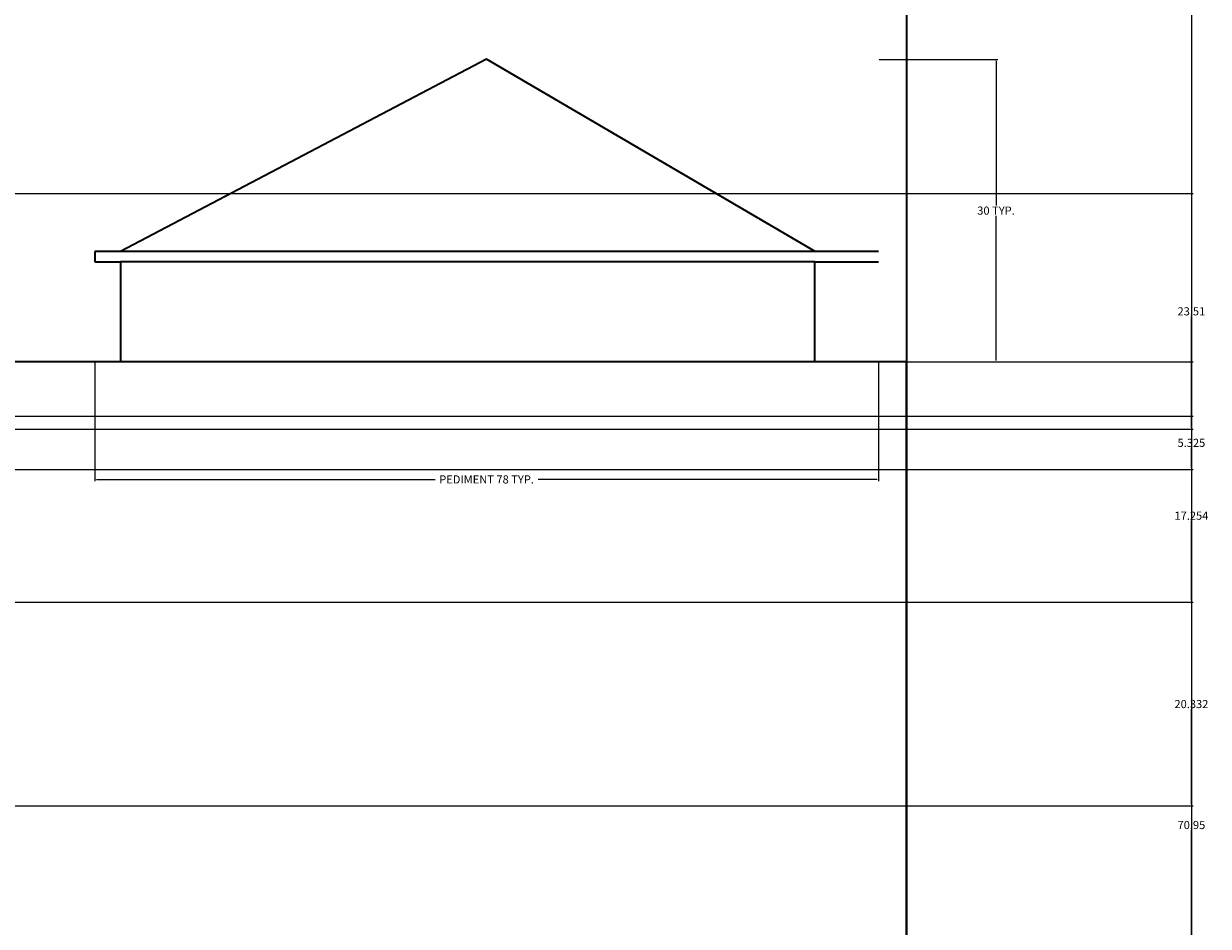
# Model space of a CAD drawing. Units: inches. Extents: x 69 to 650, y -16 to 573.
# Tile 22 of 26: x 531 to 650, y 308 to 398. Entities that reach past the tile are written whole.
import ezdxf

# ---------------------------------------------------------------- set-up
doc = ezdxf.new("R2010")
doc.units = ezdxf.units.IN
doc.header["$MEASUREMENT"] = 0
for name, color, linetype, lineweight in [('A-ANNO-DIMS', 2, 'Continuous', 18), ('A-ROOF', 7, 'Continuous', 35), ('A-WALL', 7, 'Continuous', 35)]:
    doc.layers.add(name, color=color, linetype=linetype, lineweight=lineweight)
doc.styles.get("Standard").update_dxf_attribs({"font": 'arial.ttf'})
doc.dimstyles.get("Standard").update_dxf_attribs({"dimtxt": 0.8125, "dimasz": 0.18, "dimexe": 0.18, "dimexo": 0.0625, "dimgap": 0.09, "dimtad": 0, "dimtih": 1, "dimtoh": 1, "dimdec": 4, "dimzin": 0, "dimdsep": 46, "dimlunit": 4, "dimtxsty": 'Standard', "dimcen": 0.09, "dimadec": 0, "dimazin": 0, "dimtfac": 1, "dimtdec": 4, "dimtofl": 0, "dimtmove": 0, "dimatfit": 3, "dimfxl": 1, "dimtolj": 1, "dimtzin": 0, "dimarcsym": 0})

# ---------------------------------------------------------------- blocks, each defined once
blk = doc.blocks.new('CAP-SIDE-PEDIMENT')
for p, q in [((39.09, 30.19), (2.58, 11)), ((71.85, 11), (39.09, 30.19)), ((78.18, 11), (0, 11)), ((0, 11), (0, 9.99)), ((0, 9.99), (2.58, 9.99)), ((71.82, 9.99), (2.58, 9.99)), ((2.58, 9.99), (2.58, 0)), ((71.82, 0), (71.82, 9.99)), ((71.82, 9.99), (78.18, 9.99))]:
    blk.add_line(p, q)
blk = doc.blocks.new('*D17')
at = {"layer": 'A-ANNO-DIMS', "color": 0, "lineweight": -2, "transparency": 16777216}
for p, q in [((538.56, 363.81), (538.56, 351.97)), ((616.75, 363.81), (616.75, 351.97)), ((538.74, 352.15), (572.52, 352.15)), ((616.57, 352.15), (582.79, 352.15))]:
    blk.add_line(p, q, dxfattribs=at)
at = {"layer": 'A-ANNO-DIMS', "color": 0, "transparency": 16777216}
for points in [[(538.74, 352.18), (538.74, 352.12), (538.56, 352.15)], [(616.57, 352.18), (616.57, 352.12), (616.75, 352.15)]]:
    blk.add_solid(points, dxfattribs=at)
at = {"layer": 'Defpoints', "color": 0, "transparency": 16777216}
for p in [(538.56, 363.87), (616.75, 363.87), (616.75, 352.15)]:
    blk.add_point(p, dxfattribs=at)
at = {"layer": 'A-ANNO-DIMS', "color": 0, "transparency": 16777216, "insert": (577.65, 352.15), "char_height": 0.8125, "attachment_point": 5}
blk.add_mtext('\\A1;PEDIMENT 78 TYP.', dxfattribs=at)
blk = doc.blocks.new('*D18')
at = {"layer": 'A-ANNO-DIMS', "color": 0, "lineweight": -2, "transparency": 16777216}
for p, q in [((616.81, 394.06), (628.65, 394.06)), ((628.47, 393.88), (628.47, 379.47)), ((628.47, 364.05), (628.47, 378.46)), ((616.81, 363.87), (628.65, 363.87))]:
    blk.add_line(p, q, dxfattribs=at)
at = {"layer": 'A-ANNO-DIMS', "color": 0, "transparency": 16777216}
for points in [[(628.44, 393.88), (628.5, 393.88), (628.47, 394.06)], [(628.44, 364.05), (628.5, 364.05), (628.47, 363.87)]]:
    blk.add_solid(points, dxfattribs=at)
at = {"layer": 'Defpoints', "color": 0, "transparency": 16777216}
for p in [(616.75, 394.06), (628.47, 394.06), (616.75, 363.87)]:
    blk.add_point(p, dxfattribs=at)
at = {"layer": 'A-ANNO-DIMS', "color": 0, "transparency": 16777216, "insert": (628.47, 378.97), "char_height": 0.8125, "attachment_point": 5}
blk.add_mtext('\\A1;30 TYP.', dxfattribs=at)
blk = doc.blocks.new('*D19')
at = {"layer": 'A-ANNO-DIMS', "color": 0, "lineweight": -2, "transparency": 16777216}
for p, q in [((99.56, 471.72), (99.56, 572.74)), ((99.74, 572.56), (358.57, 572.56)), ((619.38, 572.56), (360.54, 572.56)), ((619.56, 87.99), (619.56, 572.74))]:
    blk.add_line(p, q, dxfattribs=at)
at = {"layer": 'A-ANNO-DIMS', "color": 0, "transparency": 16777216}
for points in [[(99.74, 572.59), (99.74, 572.53), (99.56, 572.56)], [(619.38, 572.59), (619.38, 572.53), (619.56, 572.56)]]:
    blk.add_solid(points, dxfattribs=at)
at = {"layer": 'Defpoints', "color": 0, "transparency": 16777216}
for p in [(619.56, 572.56), (99.56, 471.66), (619.56, 87.93)]:
    blk.add_point(p, dxfattribs=at)
at = {"layer": 'A-ANNO-DIMS', "color": 0, "transparency": 16777216, "insert": (359.56, 572.56), "char_height": 0.812, "attachment_point": 5}
blk.add_mtext('\\A1;520', dxfattribs=at)
blk = doc.blocks.new('*D20')
at = {"layer": 'A-ANNO-DIMS', "color": 0, "lineweight": -2, "transparency": 16777216}
for p, q in [((504.24, 544.16), (648.14, 544.16)), ((647.96, 543.98), (647.96, 304.55)), ((647.96, 64.11), (647.96, 303.54)), ((619.62, 63.93), (648.14, 63.93))]:
    blk.add_line(p, q, dxfattribs=at)
at = {"layer": 'A-ANNO-DIMS', "color": 0, "transparency": 16777216}
for points in [[(647.93, 543.98), (647.99, 543.98), (647.96, 544.16)], [(647.93, 64.11), (647.99, 64.11), (647.96, 63.93)]]:
    blk.add_solid(points, dxfattribs=at)
at = {"layer": 'Defpoints', "color": 0, "transparency": 16777216}
for p in [(504.18, 544.16), (647.96, 544.16), (619.56, 63.93)]:
    blk.add_point(p, dxfattribs=at)
at = {"layer": 'A-ANNO-DIMS', "color": 0, "transparency": 16777216, "insert": (647.96, 304.04), "char_height": 0.812, "attachment_point": 5}
blk.add_mtext('\\A1;480.2', dxfattribs=at)
blk = doc.blocks.new('*D43')
at = {"layer": 'A-ANNO-DIMS', "color": 0, "lineweight": -2, "transparency": 16777216}
for p, q in [((502.63, 353.14), (648.14, 353.14)), ((647.96, 352.96), (647.96, 318.17)), ((647.96, 282.37), (647.96, 317.16)), ((502.63, 282.19), (648.14, 282.19))]:
    blk.add_line(p, q, dxfattribs=at)
at = {"layer": 'A-ANNO-DIMS', "color": 0, "transparency": 16777216}
for points in [[(647.93, 352.96), (647.99, 352.96), (647.96, 353.14)], [(647.93, 282.37), (647.99, 282.37), (647.96, 282.19)]]:
    blk.add_solid(points, dxfattribs=at)
at = {"layer": 'Defpoints', "color": 0, "transparency": 16777216}
for p in [(502.56, 353.14), (647.96, 353.14), (502.56, 282.19)]:
    blk.add_point(p, dxfattribs=at)
at = {"layer": 'A-ANNO-DIMS', "color": 0, "transparency": 16777216, "insert": (647.96, 317.67), "char_height": 0.812, "attachment_point": 5}
blk.add_mtext('\\A1;70.95', dxfattribs=at)
blk = doc.blocks.new('*D44')
at = {"layer": 'A-ANNO-DIMS', "color": 0, "lineweight": -2, "transparency": 16777216}
for p, q in [((470.47, 358.46), (648.14, 358.46)), ((647.96, 358.28), (647.96, 356.31)), ((647.96, 353.32), (647.96, 355.3)), ((502.63, 353.14), (648.14, 353.14))]:
    blk.add_line(p, q, dxfattribs=at)
at = {"layer": 'A-ANNO-DIMS', "color": 0, "transparency": 16777216}
for points in [[(647.93, 358.28), (647.99, 358.28), (647.96, 358.46)], [(647.93, 353.32), (647.99, 353.32), (647.96, 353.14)]]:
    blk.add_solid(points, dxfattribs=at)
at = {"layer": 'Defpoints', "color": 0, "transparency": 16777216}
for p in [(470.41, 358.46), (647.96, 358.46), (502.56, 353.14)]:
    blk.add_point(p, dxfattribs=at)
at = {"layer": 'A-ANNO-DIMS', "color": 0, "transparency": 16777216, "insert": (647.96, 355.8), "char_height": 0.812, "attachment_point": 5}
blk.add_mtext('\\A1;5.325', dxfattribs=at)
blk = doc.blocks.new('*D46')
at = {"layer": 'A-ANNO-DIMS', "color": 0, "lineweight": -2, "transparency": 16777216}
for p, q in [((619.62, 363.87), (648.14, 363.87)), ((647.96, 363.69), (647.96, 304.41)), ((647.96, 244.11), (647.96, 303.4)), ((619.62, 243.93), (648.14, 243.93))]:
    blk.add_line(p, q, dxfattribs=at)
at = {"layer": 'A-ANNO-DIMS', "color": 0, "transparency": 16777216}
for points in [[(647.93, 363.69), (647.99, 363.69), (647.96, 363.87)], [(647.93, 244.11), (647.99, 244.11), (647.96, 243.93)]]:
    blk.add_solid(points, dxfattribs=at)
at = {"layer": 'Defpoints', "color": 0, "transparency": 16777216}
for p in [(619.56, 363.87), (647.96, 363.87), (619.56, 243.93)]:
    blk.add_point(p, dxfattribs=at)
at = {"layer": 'A-ANNO-DIMS', "color": 0, "transparency": 16777216, "insert": (647.96, 303.9), "char_height": 0.812, "attachment_point": 5}
blk.add_mtext('\\A1;119.94', dxfattribs=at)
blk = doc.blocks.new('*D73')
at = {"layer": 'A-ANNO-DIMS', "color": 0, "lineweight": -2, "transparency": 16777216}
for p, q in [((383.36, 319.57), (648.14, 319.57)), ((647.96, 319.39), (647.96, 302.7)), ((647.96, 284.99), (647.96, 301.69)), ((383.36, 284.81), (648.14, 284.81))]:
    blk.add_line(p, q, dxfattribs=at)
at = {"layer": 'A-ANNO-DIMS', "color": 0, "transparency": 16777216}
for points in [[(647.93, 319.39), (647.99, 319.39), (647.96, 319.57)], [(647.93, 284.99), (647.99, 284.99), (647.96, 284.81)]]:
    blk.add_solid(points, dxfattribs=at)
at = {"layer": 'Defpoints', "color": 0, "transparency": 16777216}
for p in [(383.3, 319.57), (647.96, 319.57), (383.3, 284.81)]:
    blk.add_point(p, dxfattribs=at)
at = {"layer": 'A-ANNO-DIMS', "color": 0, "transparency": 16777216, "insert": (647.96, 302.19), "char_height": 0.812, "attachment_point": 5}
blk.add_mtext('\\A1;34.76', dxfattribs=at)
blk = doc.blocks.new('*D74')
at = {"layer": 'A-ANNO-DIMS', "color": 0, "lineweight": -2, "transparency": 16777216}
for p, q in [((383.36, 339.91), (648.14, 339.91)), ((647.96, 339.73), (647.96, 330.25)), ((647.96, 319.75), (647.96, 329.23)), ((383.36, 319.57), (648.14, 319.57))]:
    blk.add_line(p, q, dxfattribs=at)
at = {"layer": 'A-ANNO-DIMS', "color": 0, "transparency": 16777216}
for points in [[(647.93, 339.73), (647.99, 339.73), (647.96, 339.91)], [(647.93, 319.75), (647.99, 319.75), (647.96, 319.57)]]:
    blk.add_solid(points, dxfattribs=at)
at = {"layer": 'Defpoints', "color": 0, "transparency": 16777216}
for p in [(383.3, 339.91), (647.96, 339.91), (383.3, 319.57)]:
    blk.add_point(p, dxfattribs=at)
at = {"layer": 'A-ANNO-DIMS', "color": 0, "transparency": 16777216, "insert": (647.96, 329.74), "char_height": 0.812, "attachment_point": 5}
blk.add_mtext('\\A1;20.332', dxfattribs=at)
blk = doc.blocks.new('*D75')
at = {"layer": 'A-ANNO-DIMS', "color": 0, "lineweight": -2, "transparency": 16777216}
for p, q in [((383.36, 357.16), (648.14, 357.16)), ((647.96, 356.98), (647.96, 349.04)), ((647.96, 340.09), (647.96, 348.03)), ((383.36, 339.91), (648.14, 339.91))]:
    blk.add_line(p, q, dxfattribs=at)
at = {"layer": 'A-ANNO-DIMS', "color": 0, "transparency": 16777216}
for points in [[(647.93, 356.98), (647.99, 356.98), (647.96, 357.16)], [(647.93, 340.09), (647.99, 340.09), (647.96, 339.91)]]:
    blk.add_solid(points, dxfattribs=at)
at = {"layer": 'Defpoints', "color": 0, "transparency": 16777216}
for p in [(383.3, 357.16), (647.96, 357.16), (383.3, 339.91)]:
    blk.add_point(p, dxfattribs=at)
at = {"layer": 'A-ANNO-DIMS', "color": 0, "transparency": 16777216, "insert": (647.96, 348.53), "char_height": 0.812, "attachment_point": 5}
blk.add_mtext('\\A1;17.254', dxfattribs=at)
blk = doc.blocks.new('*D76')
at = {"layer": 'A-ANNO-DIMS', "color": 0, "lineweight": -2, "transparency": 16777216}
for p, q in [((383.36, 380.67), (648.14, 380.67)), ((647.96, 380.49), (647.96, 369.42)), ((647.96, 357.34), (647.96, 368.41)), ((383.36, 357.16), (648.14, 357.16))]:
    blk.add_line(p, q, dxfattribs=at)
at = {"layer": 'A-ANNO-DIMS', "color": 0, "transparency": 16777216}
for points in [[(647.93, 380.49), (647.99, 380.49), (647.96, 380.67)], [(647.93, 357.34), (647.99, 357.34), (647.96, 357.16)]]:
    blk.add_solid(points, dxfattribs=at)
at = {"layer": 'Defpoints', "color": 0, "transparency": 16777216}
for p in [(383.3, 380.67), (647.96, 380.67), (383.3, 357.16)]:
    blk.add_point(p, dxfattribs=at)
at = {"layer": 'A-ANNO-DIMS', "color": 0, "transparency": 16777216, "insert": (647.96, 368.92), "char_height": 0.812, "attachment_point": 5}
blk.add_mtext('\\A1;23.51', dxfattribs=at)

msp = doc.modelspace()

# ---------------------------------------------------------------- linework, layer by layer
at = {"layer": 'A-WALL'}
msp.add_line((619.555, 411.93), (619.555, 69.3788), dxfattribs=at)
msp.add_lwpolyline([(619.555, 363.8739), (528.812, 363.8739), (528.812, 243.93), (619.555, 243.93)], close=True, dxfattribs=at)

# ---------------------------------------------------------------- block references
at = {"layer": 'A-ROOF'}
msp.add_blockref('CAP-SIDE-PEDIMENT', (538.563, 363.874), dxfattribs=at)

# ---------------------------------------------------------------- dimensions: what is measured, and where the dimension line sits
at = {"layer": 'A-ANNO-DIMS'}
dim = msp.add_linear_dim(base=(619.555, 572.5573), p1=(99.556, 471.6595), p2=(619.555, 87.93), dimstyle='Standard', override={"dimdec": 0, "dimlfac": 1, "dimrnd": 0, "dimzin": 0, "dimdsep": 46, "dimlunit": 2}, dxfattribs=at)
dim.commit()
dim.dimension.update_dxf_attribs({"geometry": '*D19', "text_midpoint": (359.5555, 572.5573)})
for base, p1, p2, override, picture, middle in [((647.955, 544.1573), (619.555, 63.93), (504.1763, 544.1573), {"dimdec": 1, "dimlfac": 1, "dimrnd": 0, "dimzin": 0, "dimdsep": 46, "dimlunit": 2}, '*D20', (647.955, 304.0436)), ((647.955, 380.6715), (383.3022, 357.1599), (383.3022, 380.6715), {"dimdec": 2, "dimlfac": 1, "dimrnd": 0, "dimzin": 0, "dimdsep": 46, "dimlunit": 2}, '*D76', (647.955, 368.9157)), ((647.955, 363.8739), (619.555, 243.93), (619.555, 363.8739), {"dimdec": 2, "dimlfac": 1, "dimrnd": 0, "dimzin": 0, "dimdsep": 46, "dimlunit": 2}, '*D46', (647.955, 303.902)), ((647.955, 358.4634), (502.5637, 353.1381), (470.4053, 358.4634), {"dimdec": 3, "dimlfac": 1, "dimrnd": 0, "dimzin": 0, "dimdsep": 46, "dimlunit": 2}, '*D44', (647.955, 355.8008)), ((647.955, 357.1599), (383.3022, 339.9061), (383.3022, 357.1599), {"dimdec": 3, "dimlfac": 1, "dimrnd": 0, "dimzin": 0, "dimdsep": 46, "dimlunit": 2}, '*D75', (647.955, 348.533)), ((647.955, 353.1381), (502.5637, 282.1923), (502.5637, 353.1381), {"dimdec": 2, "dimlfac": 1, "dimrnd": 0, "dimzin": 0, "dimdsep": 46, "dimlunit": 2}, '*D43', (647.955, 317.6652)), ((647.955, 339.9061), (383.3022, 319.5737), (383.3022, 339.9061), {"dimdec": 3, "dimlfac": 1, "dimrnd": 0, "dimzin": 0, "dimdsep": 46, "dimlunit": 2}, '*D74', (647.955, 329.7399)), ((647.955, 319.5737), (383.3022, 284.812), (383.3022, 319.5737), {"dimdec": 2, "dimlfac": 1, "dimrnd": 0, "dimzin": 0, "dimdsep": 46, "dimlunit": 2}, '*D73', (647.955, 302.1928))]:
    dim = msp.add_linear_dim(base=base, p1=p1, p2=p2, angle=90, dimstyle='Standard', override=override, dxfattribs=at)
    dim.commit()
    dim.dimension.update_dxf_attribs({"geometry": picture, "text_midpoint": middle})
dim = msp.add_linear_dim(base=(628.4729, 394.063), p1=(616.7456, 363.8739), p2=(616.7456, 394.063), angle=90, text='<> TYP.', dimstyle='Standard', override={"dimdec": 0, "dimlfac": 1, "dimrnd": 0, "dimzin": 0, "dimdsep": 46, "dimlunit": 2}, dxfattribs=at)
dim.commit()
dim.dimension.update_dxf_attribs({"geometry": '*D18', "text_midpoint": (628.4729, 378.9685)})
dim = msp.add_linear_dim(base=(616.7456, 352.1466), p1=(538.5634, 363.8739), p2=(616.7456, 363.8739), text='PEDIMENT <> TYP.', dimstyle='Standard', override={"dimdec": 0, "dimlfac": 1, "dimrnd": 0, "dimzin": 0, "dimdsep": 46, "dimlunit": 2}, dxfattribs=at)
dim.commit()
dim.dimension.update_dxf_attribs({"geometry": '*D17', "text_midpoint": (577.6545, 352.1466)})

doc.saveas('drawing.dxf')
